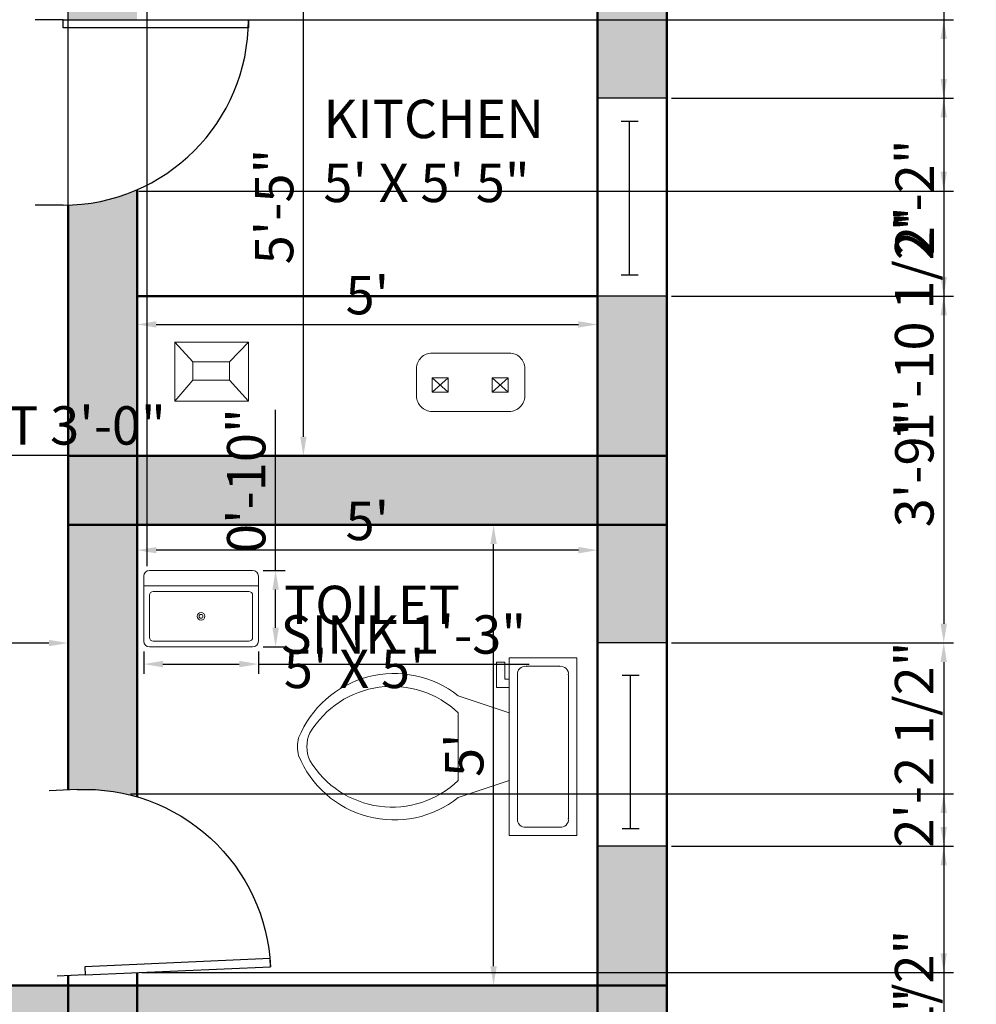
# Model space of a CAD drawing. Units: millimetres. Extents: x 2784 to 3697, y 603 to 1406.
# Tile 6 of 10: x 3091 to 3215, y 1077 to 1205. Entities that reach past the tile are written whole.
import ezdxf

# ---------------------------------------------------------------- set-up
doc = ezdxf.new("R2010")
doc.units = ezdxf.units.MM
for name, color, linetype, lineweight in [('A-ANNO-DIMS', 140, 'Continuous', 18), ('A-AREA-IDEN', 150, 'Continuous', 25), ('A-DOOR', 10, 'Continuous', 25), ('A-FLOR-FIXT', 8, 'Continuous', 18), ('A-FURN', 80, 'Continuous', 18), ('A-GLAZ', 30, 'Continuous', 25), ('A-WALL', 2, 'Continuous', 50), ('A-WALL-PATT', 8, 'Continuous', 13)]:
    doc.layers.add(name, color=color, linetype=linetype, lineweight=lineweight)
doc.styles.get("Standard").update_dxf_attribs({"font": 'arial.ttf'})
doc.dimstyles.new('ISO-25', dxfattribs={"dimtxt": 5, "dimasz": 2.5, "dimexe": 1.25, "dimexo": 0.625, "dimtad": 1, "dimdec": 0, "dimlunit": 3, "dimtxsty": 'Standard', "dimcen": 2.5, "dimadec": 0, "dimazin": 0, "dimtfac": 1, "dimtdec": 0, "dimtmove": 0, "dimatfit": 3, "dimfxl": 1, "dimarcsym": 0})

# ---------------------------------------------------------------- blocks, each defined once
blk = doc.blocks.new('*U2')
for p, q in [((0, 0), (0, -6)), ((40, 0), (40, -6))]:
    blk.add_line(p, q)
blk.add_lwpolyline([(0, 0), (0, 40), (1.75, 40), (1.75, 0)], close=True)
blk.add_arc((0, 0), 40, 0, 90)
blk = doc.blocks.new('*U5')
for p, q in [((0, 4), (0, 0)), ((36, 4), (36, 0)), ((0, 2), (36, 2))]:
    blk.add_line(p, q)
blk = doc.blocks.new('Toilet - top')
for p, q in [((9.5, -6), (9.5, -2)), ((-8, -8.5), (-8, -8)), ((-7, -8), (-7, -9.5)), ((-4, -8), (-6, -14)), ((4, -8), (6, -14)), ((-10, -8.5), (-8, -8.5)), ((-10, -9.5), (-10, -8.5)), ((-7, -9.5), (-10, -9.5)), ((4, -14), (-4, -14))]:
    blk.add_line(p, q)
blk.add_lwpolyline([(10.5, -8), (10.5, 0), (-10.5, 0), (-10.5, -8)], close=True)
for points in [[(8.5, -1), (-8.5, -1)], [(-9.5, -2), (-9.5, -6)], [(-8.5, -7), (8.5, -7)]]:
    blk.add_lwpolyline(points)
for centre, radius, start, end in [((-8.62, -1.88), 0.884, 81.8699, 188.1301), ((8.62, -1.88), 0.884, 351.8699, 98.1301), ((-8.62, -6.12), 0.884, 171.8699, 278.1301), ((8.62, -6.12), 0.884, 261.8699, 8.1301), ((3.52, -21.58), 12.17, 141.4691, 247.9714), ((4.2, -21.82), 11.33, 136.3677, 238.9468), ((-3.52, -21.58), 12.17, 292.0284, 38.5307), ((-4.2, -21.82), 11.33, 301.053, 43.6321), ((0, -27.88), 4, 245.7318, 294.2682), ((0, -29), 4, 254.8605, 285.1395)]:
    blk.add_arc(centre, radius, start, end)
blk = doc.blocks.new('Sink-single - 30 in top')
blk.add_line((-15, -3.999996), (15, -3.999996))
for points in [[(-13.5, 0), (13.5, 0)], [(-15, -18.499996), (-15, -1.5)], [(15, -1.5), (15, -18.499996)], [(-13.5, -17.499996), (-13.5, -6.499996)], [(-12.5, -5.499996), (12.5, -5.499996)], [(13.5, -6.499996), (13.5, -17.499996)], [(13.5, -19.999996), (-13.5, -19.999996)], [(12.5, -18.499996), (-12.5, -18.499996)]]:
    blk.add_lwpolyline(points)
for radius in [1, 0.5]:
    blk.add_circle((0, -11.999996), radius)
for centre, radius, start, end in [((-13.5, -1.5), 1.5, 90, 180), ((13.5, -1.5), 1.5, 0, 90), ((-12.5, -6.499996), 1, 90, 180), ((12.5, -6.499996), 1, 0, 90), ((-12.5, -17.499996), 1, 180, 270), ((12.5, -17.499996), 1, 270, 0), ((-13.5, -18.499996), 1.5, 180, 270), ((13.5, -18.499996), 1.5, 270, 0)]:
    blk.add_arc(centre, radius, start, end)
blk = doc.blocks.new('*D23')
at = {"layer": 'A-ANNO-DIMS', "color": 0, "lineweight": -2, "transparency": 16777216}
for p, q in [((3105.91, 1165.32), (3105.91, 1164.11)), ((3108.41, 1165.36), (3163.41, 1165.36)), ((3165.91, 1165.32), (3165.91, 1164.11))]:
    blk.add_line(p, q, dxfattribs=at)
at = {"layer": 'A-ANNO-DIMS', "color": 0, "transparency": 16777216}
for points in [[(3108.41, 1165.78), (3108.41, 1164.95), (3105.91, 1165.36)], [(3163.41, 1165.78), (3163.41, 1164.95), (3165.91, 1165.36)]]:
    blk.add_solid(points, dxfattribs=at)
at = {"layer": 'Defpoints', "color": 0, "transparency": 16777216}
for p in [(3105.91, 1165.95), (3165.91, 1165.95), (3165.91, 1165.36)]:
    blk.add_point(p, dxfattribs=at)
at = {"layer": 'A-ANNO-DIMS', "color": 0, "transparency": 16777216, "insert": (3135.91, 1168.53), "char_height": 5, "attachment_point": 5}
blk.add_mtext("5'", dxfattribs=at)
blk = doc.blocks.new('*D24')
at = {"layer": 'A-ANNO-DIMS', "color": 0, "lineweight": -2, "transparency": 16777216}
for p, q in [((3124.34, 1213.23), (3128.82, 1213.23)), ((3127.57, 1150.73), (3127.57, 1210.73)), ((3124.34, 1148.23), (3128.82, 1148.23))]:
    blk.add_line(p, q, dxfattribs=at)
at = {"layer": 'A-ANNO-DIMS', "color": 0, "transparency": 16777216}
for points in [[(3127.15, 1210.73), (3127.98, 1210.73), (3127.57, 1213.23)], [(3127.15, 1150.73), (3127.98, 1150.73), (3127.57, 1148.23)]]:
    blk.add_solid(points, dxfattribs=at)
at = {"layer": 'Defpoints', "color": 0, "transparency": 16777216}
for p in [(3123.72, 1213.23), (3127.57, 1213.23), (3123.72, 1148.23)]:
    blk.add_point(p, dxfattribs=at)
at = {"layer": 'A-ANNO-DIMS', "color": 0, "transparency": 16777216, "insert": (3124.4, 1180.73), "char_height": 5, "attachment_point": 5, "rotation": 90}
blk.add_mtext('5\'-5"', dxfattribs=at)
blk = doc.blocks.new('*D25')
at = {"layer": 'A-ANNO-DIMS', "color": 0, "lineweight": -2, "transparency": 16777216}
for p, q in [((3105.91, 1136.2), (3105.91, 1134.7)), ((3163.41, 1135.95), (3108.41, 1135.95)), ((3165.91, 1136.2), (3165.91, 1134.7))]:
    blk.add_line(p, q, dxfattribs=at)
at = {"layer": 'A-ANNO-DIMS', "color": 0, "transparency": 16777216}
for points in [[(3108.41, 1136.36), (3108.41, 1135.53), (3105.91, 1135.95)], [(3163.41, 1136.36), (3163.41, 1135.53), (3165.91, 1135.95)]]:
    blk.add_solid(points, dxfattribs=at)
at = {"layer": 'Defpoints', "color": 0, "transparency": 16777216}
for p in [(3105.91, 1136.83), (3165.91, 1136.83), (3105.91, 1135.95)]:
    blk.add_point(p, dxfattribs=at)
at = {"layer": 'A-ANNO-DIMS', "color": 0, "transparency": 16777216, "insert": (3135.91, 1139.11), "char_height": 5, "attachment_point": 5}
blk.add_mtext("5'", dxfattribs=at)
blk = doc.blocks.new('*D26')
at = {"layer": 'A-ANNO-DIMS', "color": 0, "lineweight": -2, "transparency": 16777216}
for p, q in [((3152.97, 1139.23), (3153.6, 1139.23)), ((3152.35, 1081.73), (3152.35, 1136.73)), ((3152.97, 1079.23), (3153.6, 1079.23))]:
    blk.add_line(p, q, dxfattribs=at)
at = {"layer": 'A-ANNO-DIMS', "color": 0, "transparency": 16777216}
for points in [[(3151.93, 1136.73), (3152.77, 1136.73), (3152.35, 1139.23)], [(3151.93, 1081.73), (3152.77, 1081.73), (3152.35, 1079.23)]]:
    blk.add_solid(points, dxfattribs=at)
at = {"layer": 'Defpoints', "color": 0, "transparency": 16777216}
for p in [(3152.35, 1139.23), (3152.35, 1139.23), (3152.35, 1079.23)]:
    blk.add_point(p, dxfattribs=at)
at = {"layer": 'A-ANNO-DIMS', "color": 0, "transparency": 16777216, "insert": (3149.18, 1109.23), "char_height": 5, "attachment_point": 5, "rotation": 90}
blk.add_mtext("5'", dxfattribs=at)
blk = doc.blocks.new('*D36')
at = {"layer": 'A-ANNO-DIMS', "color": 0, "lineweight": -2, "transparency": 16777216}
for p, q in [((2971.91, 1166.33), (2971.91, 1122.59)), ((3096.91, 1166.33), (3096.91, 1122.59)), ((3094.41, 1123.84), (2974.41, 1123.84))]:
    blk.add_line(p, q, dxfattribs=at)
at = {"layer": 'A-ANNO-DIMS', "color": 0, "transparency": 16777216}
for points in [[(2974.41, 1124.26), (2974.41, 1123.43), (2971.91, 1123.84)], [(3094.41, 1124.26), (3094.41, 1123.43), (3096.91, 1123.84)]]:
    blk.add_solid(points, dxfattribs=at)
at = {"layer": 'Defpoints', "color": 0, "transparency": 16777216}
for p in [(2971.91, 1166.96), (3096.91, 1166.96), (2971.91, 1123.84)]:
    blk.add_point(p, dxfattribs=at)
at = {"layer": 'A-ANNO-DIMS', "color": 0, "transparency": 16777216, "insert": (3034.41, 1127.02), "char_height": 5, "attachment_point": 5}
blk.add_mtext('10\'-5"', dxfattribs=at)
blk = doc.blocks.new('*D66')
at = {"layer": 'A-ANNO-DIMS', "color": 0, "lineweight": -2, "transparency": 16777216}
for p, q in [((3106.77, 1122.72), (3106.77, 1119.85)), ((3121.71, 1122.72), (3121.71, 1119.85)), ((3109.27, 1121.1), (3119.21, 1121.1)), ((3121.71, 1121.1), (3156.97, 1121.1))]:
    blk.add_line(p, q, dxfattribs=at)
at = {"layer": 'A-ANNO-DIMS', "color": 0, "transparency": 16777216}
for points in [[(3109.27, 1121.52), (3109.27, 1120.68), (3106.77, 1121.1)], [(3119.21, 1121.52), (3119.21, 1120.68), (3121.71, 1121.1)]]:
    blk.add_solid(points, dxfattribs=at)
at = {"layer": 'Defpoints', "color": 0, "transparency": 16777216}
for p in [(3106.77, 1123.34), (3121.71, 1123.34), (3121.71, 1121.1)]:
    blk.add_point(p, dxfattribs=at)
at = {"layer": 'A-ANNO-DIMS', "color": 0, "transparency": 16777216, "insert": (3140.59, 1124.31), "char_height": 5, "attachment_point": 5}
blk.add_mtext('SINK 1\'-3"', dxfattribs=at)
blk = doc.blocks.new('*D67')
at = {"layer": 'A-ANNO-DIMS', "color": 0, "lineweight": -2, "transparency": 16777216}
for p, q in [((3123.95, 1133.3), (3123.95, 1154.22)), ((3122.33, 1133.3), (3125.2, 1133.3)), ((3123.95, 1125.84), (3123.95, 1130.8)), ((3122.33, 1123.34), (3125.2, 1123.34))]:
    blk.add_line(p, q, dxfattribs=at)
at = {"layer": 'A-ANNO-DIMS', "color": 0, "transparency": 16777216}
for points in [[(3123.53, 1130.8), (3124.37, 1130.8), (3123.95, 1133.3)], [(3123.53, 1125.84), (3124.37, 1125.84), (3123.95, 1123.34)]]:
    blk.add_solid(points, dxfattribs=at)
at = {"layer": 'Defpoints', "color": 0, "transparency": 16777216}
for p in [(3121.71, 1133.3), (3123.95, 1133.3), (3121.71, 1123.34)]:
    blk.add_point(p, dxfattribs=at)
at = {"layer": 'A-ANNO-DIMS', "color": 0, "transparency": 16777216, "insert": (3120.77, 1145.01), "char_height": 5, "attachment_point": 5, "rotation": 90}
blk.add_mtext('0\'-10"', dxfattribs=at)
blk = doc.blocks.new('*D74')
at = {"layer": 'A-ANNO-DIMS', "color": 0, "lineweight": -2, "transparency": 16777216}
for p, q in [((3016.17, 1153.13), (3016.17, 1147.09)), ((3052.27, 1153.13), (3052.27, 1147.09)), ((3018.67, 1148.34), (3049.77, 1148.34)), ((3052.27, 1148.34), (3110.98, 1148.34))]:
    blk.add_line(p, q, dxfattribs=at)
at = {"layer": 'A-ANNO-DIMS', "color": 0, "transparency": 16777216}
for points in [[(3018.67, 1148.76), (3018.67, 1147.92), (3016.17, 1148.34)], [(3049.77, 1148.76), (3049.77, 1147.92), (3052.27, 1148.34)]]:
    blk.add_solid(points, dxfattribs=at)
at = {"layer": 'Defpoints', "color": 0, "transparency": 16777216}
for p in [(3016.17, 1153.76), (3052.27, 1153.76), (3052.27, 1148.34)]:
    blk.add_point(p, dxfattribs=at)
at = {"layer": 'A-ANNO-DIMS', "color": 0, "transparency": 16777216, "insert": (3082.87, 1151.55), "char_height": 5, "attachment_point": 5}
blk.add_mtext('DINING SET 3\'-0"', dxfattribs=at)
blk = doc.blocks.new('*D93')
at = {"layer": 'A-ANNO-DIMS', "color": 0, "lineweight": -2, "transparency": 16777216}
for p, q in [((3175.53, 1266.65), (3212.26, 1266.65)), ((3211.01, 1264.15), (3211.01, 1197.33)), ((3175.53, 1194.83), (3212.26, 1194.83))]:
    blk.add_line(p, q, dxfattribs=at)
at = {"layer": 'A-ANNO-DIMS', "color": 0, "transparency": 16777216}
for points in [[(3210.59, 1264.15), (3211.42, 1264.15), (3211.01, 1266.65)], [(3210.59, 1197.33), (3211.42, 1197.33), (3211.01, 1194.83)]]:
    blk.add_solid(points, dxfattribs=at)
at = {"layer": 'Defpoints', "color": 0, "transparency": 16777216}
for p in [(3174.91, 1266.65), (3174.91, 1194.83), (3211.01, 1194.83)]:
    blk.add_point(p, dxfattribs=at)
at = {"layer": 'A-ANNO-DIMS', "color": 0, "transparency": 16777216, "insert": (3207.83, 1230.74), "char_height": 5, "attachment_point": 5, "rotation": 90}
blk.add_mtext('6\'-0"', dxfattribs=at)
blk = doc.blocks.new('*D94')
at = {"layer": 'A-ANNO-DIMS', "color": 0, "lineweight": -2, "transparency": 16777216}
for p, q in [((3175.53, 1194.83), (3212.26, 1194.83)), ((3211.01, 1192.33), (3211.01, 1171.56)), ((3175.53, 1169.06), (3212.26, 1169.06))]:
    blk.add_line(p, q, dxfattribs=at)
at = {"layer": 'A-ANNO-DIMS', "color": 0, "transparency": 16777216}
for points in [[(3210.59, 1192.33), (3211.42, 1192.33), (3211.01, 1194.83)], [(3210.59, 1171.56), (3211.42, 1171.56), (3211.01, 1169.06)]]:
    blk.add_solid(points, dxfattribs=at)
at = {"layer": 'Defpoints', "color": 0, "transparency": 16777216}
for p in [(3174.91, 1194.83), (3174.91, 1169.06), (3211.01, 1169.06)]:
    blk.add_point(p, dxfattribs=at)
at = {"layer": 'A-ANNO-DIMS', "color": 0, "transparency": 16777216, "insert": (3207.87, 1181.94), "char_height": 5, "attachment_point": 5, "rotation": 90}
blk.add_mtext('2\'-2"', dxfattribs=at)
blk = doc.blocks.new('*D95')
at = {"layer": 'A-ANNO-DIMS', "color": 0, "lineweight": -2, "transparency": 16777216}
for p, q in [((3175.53, 1169.06), (3212.26, 1169.06)), ((3211.01, 1166.56), (3211.01, 1126.36)), ((3175.53, 1123.86), (3212.26, 1123.86))]:
    blk.add_line(p, q, dxfattribs=at)
at = {"layer": 'A-ANNO-DIMS', "color": 0, "transparency": 16777216}
for points in [[(3210.59, 1166.56), (3211.42, 1166.56), (3211.01, 1169.06)], [(3210.59, 1126.36), (3211.42, 1126.36), (3211.01, 1123.86)]]:
    blk.add_solid(points, dxfattribs=at)
at = {"layer": 'Defpoints', "color": 0, "transparency": 16777216}
for p in [(3174.91, 1169.06), (3174.91, 1123.86), (3211.01, 1123.86)]:
    blk.add_point(p, dxfattribs=at)
at = {"layer": 'A-ANNO-DIMS', "color": 0, "transparency": 16777216, "insert": (3207.83, 1146.46), "char_height": 5, "attachment_point": 5, "rotation": 90}
blk.add_mtext('3\'-9"', dxfattribs=at)
blk = doc.blocks.new('*D96')
at = {"layer": 'A-ANNO-DIMS', "color": 0, "lineweight": -2, "transparency": 16777216}
for p, q in [((3175.53, 1123.86), (3212.26, 1123.86)), ((3211.01, 1121.36), (3211.01, 1099.87)), ((3175.53, 1097.37), (3212.26, 1097.37))]:
    blk.add_line(p, q, dxfattribs=at)
at = {"layer": 'A-ANNO-DIMS', "color": 0, "transparency": 16777216}
for points in [[(3210.59, 1121.36), (3211.42, 1121.36), (3211.01, 1123.86)], [(3210.59, 1099.87), (3211.42, 1099.87), (3211.01, 1097.37)]]:
    blk.add_solid(points, dxfattribs=at)
at = {"layer": 'Defpoints', "color": 0, "transparency": 16777216}
for p in [(3174.91, 1123.86), (3174.91, 1097.37), (3211.01, 1097.37)]:
    blk.add_point(p, dxfattribs=at)
at = {"layer": 'A-ANNO-DIMS', "color": 0, "transparency": 16777216, "insert": (3207.8, 1110.61), "char_height": 5, "attachment_point": 5, "rotation": 90}
blk.add_mtext('2\'-2 1/2"', dxfattribs=at)
blk = doc.blocks.new('*D97')
at = {"layer": 'A-ANNO-DIMS', "color": 0, "lineweight": -2, "transparency": 16777216}
for p, q in [((3175.53, 1097.37), (3212.26, 1097.37)), ((3211.01, 1094.87), (3211.01, 1051.27)), ((3175.53, 1048.77), (3212.26, 1048.77))]:
    blk.add_line(p, q, dxfattribs=at)
at = {"layer": 'A-ANNO-DIMS', "color": 0, "transparency": 16777216}
for points in [[(3210.59, 1094.87), (3211.42, 1094.87), (3211.01, 1097.37)], [(3210.59, 1051.27), (3211.42, 1051.27), (3211.01, 1048.77)]]:
    blk.add_solid(points, dxfattribs=at)
at = {"layer": 'Defpoints', "color": 0, "transparency": 16777216}
for p in [(3174.91, 1097.37), (3174.91, 1048.77), (3211.01, 1048.77)]:
    blk.add_point(p, dxfattribs=at)
at = {"layer": 'A-ANNO-DIMS', "color": 0, "transparency": 16777216, "insert": (3207.8, 1073.07), "char_height": 5, "attachment_point": 5, "rotation": 90}
blk.add_mtext('4\'-0 1/2"', dxfattribs=at)
blk = doc.blocks.new('*D106')
at = {"layer": 'A-ANNO-DIMS', "color": 0, "lineweight": -2, "transparency": 16777216}
for p, q in [((3106.53, 1205.07), (3212.26, 1205.07)), ((3211.01, 1202.57), (3211.01, 1185.25)), ((3106.12, 1182.75), (3212.26, 1182.75)), ((3211.01, 1182.75), (3211.01, 1150.64))]:
    blk.add_line(p, q, dxfattribs=at)
at = {"layer": 'A-ANNO-DIMS', "color": 0, "transparency": 16777216}
for points in [[(3210.59, 1202.57), (3211.42, 1202.57), (3211.01, 1205.07)], [(3210.59, 1185.25), (3211.42, 1185.25), (3211.01, 1182.75)]]:
    blk.add_solid(points, dxfattribs=at)
at = {"layer": 'Defpoints', "color": 0, "transparency": 16777216}
for p in [(3105.91, 1205.07), (3105.49, 1182.75), (3211.01, 1182.75)]:
    blk.add_point(p, dxfattribs=at)
at = {"layer": 'A-ANNO-DIMS', "color": 0, "transparency": 16777216, "insert": (3207.8, 1165.44), "char_height": 5, "attachment_point": 5, "rotation": 90}
blk.add_mtext('1\'-10 1/2"', dxfattribs=at)
blk = doc.blocks.new('*D107')
at = {"layer": 'A-ANNO-DIMS', "color": 0, "lineweight": -2, "transparency": 16777216}
for p, q in [((3105.04, 1104.19), (3212.26, 1104.19)), ((3211.01, 1101.69), (3211.01, 1083.41)), ((3106.53, 1080.91), (3212.26, 1080.91)), ((3211.01, 1080.91), (3211.01, 1048.8))]:
    blk.add_line(p, q, dxfattribs=at)
at = {"layer": 'A-ANNO-DIMS', "color": 0, "transparency": 16777216}
for points in [[(3210.59, 1101.69), (3211.42, 1101.69), (3211.01, 1104.19)], [(3210.59, 1083.41), (3211.42, 1083.41), (3211.01, 1080.91)]]:
    blk.add_solid(points, dxfattribs=at)
at = {"layer": 'Defpoints', "color": 0, "transparency": 16777216}
for p in [(3104.41, 1104.19), (3105.91, 1080.91), (3211.01, 1080.91)]:
    blk.add_point(p, dxfattribs=at)
at = {"layer": 'A-ANNO-DIMS', "color": 0, "transparency": 16777216, "insert": (3207.8, 1063.61), "char_height": 5, "attachment_point": 5, "rotation": 90}
blk.add_mtext('1\'-11 1/2"', dxfattribs=at)
blk = doc.blocks.new('*D108')
at = {"layer": 'A-ANNO-DIMS', "color": 0, "lineweight": -2, "transparency": 16777216}
for p, q in [((3165.91, 1169.69), (3165.91, 1393.58)), ((3174.91, 1169.69), (3174.91, 1393.58)), ((3168.41, 1392.33), (3172.41, 1392.33)), ((3174.91, 1392.33), (3191.95, 1392.33))]:
    blk.add_line(p, q, dxfattribs=at)
at = {"layer": 'A-ANNO-DIMS', "color": 0, "transparency": 16777216}
for points in [[(3168.41, 1392.75), (3168.41, 1391.91), (3165.91, 1392.33)], [(3172.41, 1392.75), (3172.41, 1391.91), (3174.91, 1392.33)]]:
    blk.add_solid(points, dxfattribs=at)
at = {"layer": 'Defpoints', "color": 0, "transparency": 16777216}
for p in [(3174.91, 1392.33), (3165.91, 1169.06), (3174.91, 1169.06)]:
    blk.add_point(p, dxfattribs=at)
at = {"layer": 'A-ANNO-DIMS', "color": 0, "transparency": 16777216, "insert": (3184.68, 1395.51), "char_height": 5, "attachment_point": 5}
blk.add_mtext('0\'-9"', dxfattribs=at)
blk = doc.blocks.new('*D109')
at = {"layer": 'A-ANNO-DIMS', "color": 0, "lineweight": -2, "transparency": 16777216}
for p, q in [((3096.91, 1139.86), (3096.91, 1393.58)), ((3107.23, 1133.86), (3107.23, 1393.58)), ((3099.41, 1392.33), (3104.73, 1392.33)), ((3107.23, 1392.33), (3139.81, 1392.33))]:
    blk.add_line(p, q, dxfattribs=at)
at = {"layer": 'A-ANNO-DIMS', "color": 0, "transparency": 16777216}
for points in [[(3099.41, 1392.75), (3099.41, 1391.91), (3096.91, 1392.33)], [(3104.73, 1392.75), (3104.73, 1391.91), (3107.23, 1392.33)]]:
    blk.add_solid(points, dxfattribs=at)
at = {"layer": 'Defpoints', "color": 0, "transparency": 16777216}
for p in [(3107.23, 1392.33), (3096.91, 1139.23), (3107.23, 1133.24)]:
    blk.add_point(p, dxfattribs=at)
at = {"layer": 'A-ANNO-DIMS', "color": 0, "transparency": 16777216, "insert": (3124.77, 1395.54), "char_height": 5, "attachment_point": 5}
blk.add_mtext('0\'-10 1/2"', dxfattribs=at)

msp = doc.modelspace()

# ---------------------------------------------------------------- hatches: boundary and pattern name
at = {"layer": 'A-FLOR-FIXT'}
h = msp.add_hatch(color=256, dxfattribs=at)
h.dxf.hatch_style = 1
h.paths.add_polyline_path([(3174.91, 1169.06), (3165.91, 1169.06), (3165.91, 1148.23), (3174.91, 1148.23)])
at = {"layer": 'A-WALL-PATT'}
h = msp.add_hatch(color=256, dxfattribs=at)
h.dxf.hatch_style = 1
h.paths.add_polyline_path([(2869.53, 1356.23), (2839.91, 1356.23), (2839.91, 1347.23), (2869.53, 1347.23)])
h.paths.add_polyline_path([(2839.91, 1356.23), (2830.91, 1356.23), (2830.91, 1347.23), (2839.91, 1347.23)])
h.paths.add_polyline_path([(2839.91, 1347.23), (2830.91, 1347.23), (2830.91, 1314.23), (2839.91, 1314.23)])
h.paths.add_polyline_path([(2839.91, 1268.19), (2830.91, 1268.19), (2830.91, 1222.23), (2839.91, 1222.23)])
h.paths.add_polyline_path([(2839.91, 1222.23), (2830.91, 1222.23), (2830.91, 1213.23), (2839.91, 1213.23)])
h.paths.add_polyline_path([(2962.91, 1222.23), (2839.91, 1222.23), (2839.91, 1213.23), (2962.91, 1213.23)])
h.paths.add_polyline_path([(2971.91, 1222.23), (2962.91, 1222.23), (2962.91, 1213.23), (2971.91, 1213.23)])
h.paths.add_polyline_path([(2971.91, 1263.23), (2962.91, 1263.23), (2962.91, 1254.23), (2971.91, 1254.23)])
h.paths.add_polyline_path([(2971.91, 1347.23), (2962.91, 1347.23), (2962.91, 1263.23), (2971.91, 1263.23)])
h.paths.add_polyline_path([(2971.91, 1356.23), (2962.91, 1356.23), (2962.91, 1347.23), (2971.91, 1347.23)])
h.paths.add_polyline_path([(2962.91, 1356.23), (2913.7, 1356.23), (2913.7, 1347.23), (2962.91, 1347.23)])
h.paths.add_polyline_path([(2982.62, 1356.23), (2971.91, 1356.23), (2971.91, 1347.23), (2982.62, 1347.23)])
h.paths.add_polyline_path([(3019.91, 1356.23), (3004.44, 1356.23), (3004.44, 1347.23), (3019.91, 1347.23)])
h.paths.add_polyline_path([(3028.91, 1356.23), (3019.91, 1356.23), (3019.91, 1347.23), (3028.91, 1347.23)])
h.paths.add_polyline_path([(3028.91, 1347.23), (3019.91, 1347.23), (3019.91, 1287.35, -0.06506), (3026.12, 1288.16), (3028.91, 1288.16)])
h.paths.add_polyline_path([(3019.91, 1263.23), (2971.91, 1263.23), (2971.91, 1254.23), (3019.91, 1254.23)])
h.paths.add_polyline_path([(3028.91, 1263.23), (3019.91, 1263.23), (3019.91, 1254.23), (3028.91, 1254.23)])
h.paths.add_polyline_path([(3028.91, 1254.23), (3019.91, 1254.23), (3019.91, 1222.23), (3028.91, 1222.23)])
h.paths.add_polyline_path([(3028.91, 1222.23), (3019.91, 1222.23), (3019.91, 1213.23), (3028.91, 1213.23)])
h.paths.add_polyline_path([(3165.91, 1222.23), (3060.65, 1222.23, -0.056956), (3061.45, 1215.23), (3061.45, 1213.23), (3165.91, 1213.23)])
h.paths.add_polyline_path([(3080.34, 1356.23), (3028.91, 1356.23), (3028.91, 1347.23), (3080.34, 1347.23)])
h.paths.add_polyline_path([(3174.91, 1347.23), (3165.91, 1347.23), (3165.91, 1311.28), (3174.91, 1311.28)])
h.paths.add_polyline_path([(3174.91, 1356.23), (3165.91, 1356.23), (3165.91, 1347.23), (3174.91, 1347.23)])
h.paths.add_polyline_path([(3165.91, 1356.23), (3123.1, 1356.23), (3123.1, 1347.23), (3165.91, 1347.23)])
h.paths.add_polyline_path([(3174.91, 1266.65), (3165.91, 1266.65), (3165.91, 1222.23), (3174.91, 1222.23)])
h.paths.add_polyline_path([(3174.91, 1222.23), (3165.91, 1222.23), (3165.91, 1213.23), (3174.91, 1213.23)])
h.paths.add_polyline_path([(3174.91, 1213.23), (3165.91, 1213.23), (3165.91, 1194.83), (3174.91, 1194.83)])
h.paths.add_polyline_path([(3105.91, 1182.92, -0.096276), (3096.91, 1180.92), (3096.91, 1148.23), (3105.91, 1148.23)])
h.paths.add_polyline_path([(3105.91, 1213.23), (3096.91, 1213.23), (3096.91, 1205.07), (3105.91, 1205.07)])
h.paths.add_polyline_path([(2971.91, 1213.23), (2962.91, 1213.23), (2962.91, 1161.09), (2971.91, 1161.09)])
h.paths.add_polyline_path([(2839.91, 1213.23), (2830.91, 1213.23), (2830.91, 1157.46), (2839.91, 1157.46)])
h.paths.add_polyline_path([(2839.91, 1108.88), (2830.91, 1108.88), (2830.91, 1042.23), (2839.91, 1042.23)])
h.paths.add_polyline_path([(2839.91, 1042.23), (2830.91, 1042.23), (2830.91, 1033.23), (2839.91, 1033.23)])
h.paths.add_polyline_path([(2881.91, 1042.23), (2839.91, 1042.23), (2839.91, 1033.23), (2881.91, 1033.23)])
h.paths.add_polyline_path([(2996.91, 1042.23), (2890.91, 1042.23), (2890.91, 1033.23), (2996.91, 1033.23)])
h.paths.add_polyline_path([(2890.91, 1042.23), (2881.91, 1042.23), (2881.91, 1033.23), (2890.91, 1033.23)])
h.paths.add_polyline_path([(2890.91, 1033.23), (2881.91, 1033.23), (2881.91, 984.23), (2890.91, 984.23)])
h.paths.add_polyline_path([(2839.91, 1033.23), (2830.91, 1033.23), (2830.91, 984.23), (2839.91, 984.23)])
h.paths.add_polyline_path([(2839.91, 984.23), (2830.91, 984.23), (2830.91, 975.23), (2839.91, 975.23)])
h.paths.add_polyline_path([(2881.91, 984.23), (2854.14, 984.23, -0.154991), (2857.05, 975.23), (2881.91, 975.23)])
h.paths.add_polyline_path([(2890.91, 984.23), (2881.91, 984.23), (2881.91, 975.23), (2890.91, 975.23)])
h.paths.add_polyline_path([(2900.85, 984.23), (2890.91, 984.23), (2890.91, 975.23), (2900.85, 975.23), (2900.85, 975.78)])
h.paths.add_polyline_path([(2996.91, 984.23), (2923.49, 984.23, -0.089525), (2925.01, 975.78), (2925.01, 975.23), (2996.91, 975.23)])
h.paths.add_polyline_path([(3165.91, 984.23), (3005.91, 984.23), (3005.91, 975.23), (3165.91, 975.23)])
h.paths.add_polyline_path([(3005.91, 1033.23), (2996.91, 1033.23), (2996.91, 984.23), (3005.91, 984.23)])
h.paths.add_polyline_path([(3005.91, 984.23), (2996.91, 984.23), (2996.91, 975.23), (3005.91, 975.23)])
h.paths.add_polyline_path([(3005.91, 1042.23), (2996.91, 1042.23), (2996.91, 1033.23), (3005.91, 1033.23)])
h.paths.add_polyline_path([(3096.91, 1079.23), (2971.91, 1079.23), (2971.91, 1070.23), (3096.91, 1070.23)])
h.paths.add_polyline_path([(2971.91, 1079.23), (2962.91, 1079.23), (2962.91, 1070.23), (2971.91, 1070.23)])
h.paths.add_polyline_path([(2971.91, 1070.23), (2962.91, 1070.23), (2962.91, 1060.28, -0.115005), (2971.91, 1066.55)])
h.paths.add_polyline_path([(2971.91, 1105.54), (2962.91, 1105.54), (2962.91, 1079.23), (2971.91, 1079.23)])
h.paths.add_polyline_path([(3165.91, 1079.23), (3105.91, 1079.23), (3105.91, 1070.23), (3165.91, 1070.23)])
h.paths.add_polyline_path([(3105.91, 1079.23), (3096.91, 1079.23), (3096.91, 1070.23), (3105.91, 1070.23)])
h.paths.add_polyline_path([(3105.91, 1148.23), (3096.91, 1148.23), (3096.91, 1139.23), (3105.91, 1139.23)])
h.paths.add_polyline_path([(3105.91, 1139.23), (3096.91, 1139.23), (3096.91, 1104.7), (3098.08, 1104.75, -0.08216), (3105.91, 1103.81)])
h.paths.add_polyline_path([(3165.91, 1148.23), (3105.91, 1148.23), (3105.91, 1139.23), (3165.91, 1139.23)])
h.paths.add_polyline_path([(3174.91, 1148.23), (3165.91, 1148.23), (3165.91, 1139.23), (3174.91, 1139.23)])
h.paths.add_polyline_path([(3174.91, 1139.23), (3165.91, 1139.23), (3165.91, 1123.86), (3174.91, 1123.86)])
h.paths.add_polyline_path([(3174.91, 1097.37), (3165.91, 1097.37), (3165.91, 1079.23), (3174.91, 1079.23)])
h.paths.add_polyline_path([(3174.91, 1079.23), (3165.91, 1079.23), (3165.91, 1070.23), (3174.91, 1070.23)])
h.paths.add_polyline_path([(3174.91, 1070.23), (3165.91, 1070.23), (3165.91, 1048.77), (3174.91, 1048.77)])
h.paths.add_polyline_path([(3174.91, 1002.74), (3165.91, 1002.74), (3165.91, 984.23), (3174.91, 984.23)])
h.paths.add_polyline_path([(3174.91, 984.23), (3165.91, 984.23), (3165.91, 975.23), (3174.91, 975.23)])
h.paths.add_polyline_path([(3174.91, 975.23), (3165.91, 975.23), (3165.91, 725.23), (3174.91, 725.23)])
h.paths.add_polyline_path([(2839.91, 975.23), (2830.91, 975.23), (2830.91, 725.23), (2839.91, 725.23)])
h.paths.add_polyline_path([(3165.91, 725.23), (2839.91, 725.23), (2839.91, 716.23), (3165.91, 716.23)])
h.paths.add_polyline_path([(3174.91, 725.23), (3165.91, 725.23), (3165.91, 716.23), (3174.91, 716.23)])
h.paths.add_polyline_path([(2839.91, 725.23), (2830.91, 725.23), (2830.91, 716.23), (2839.91, 716.23)])

# ---------------------------------------------------------------- linework, layer by layer
at = {"layer": 'A-FURN'}
for p, q in [((3113.17, 1160.47), (3110.8, 1163.06)), ((3117.96, 1160.47), (3120.42, 1163.06)), ((3113.17, 1158.11), (3110.8, 1155.35)), ((3117.96, 1158.11), (3120.42, 1155.35)), ((3146.45, 1156.55), (3144.36, 1158.41)), ((3144.36, 1156.55), (3146.45, 1158.41)), ((3152.18, 1158.41), (3154.26, 1156.55)), ((3152.18, 1156.55), (3154.26, 1158.41))]:
    msp.add_line(p, q, dxfattribs=at)
for points in [[(3110.8, 1163.06), (3120.42, 1163.06), (3120.42, 1155.35), (3110.8, 1155.35)], [(3113.17, 1160.47), (3117.96, 1160.47), (3117.96, 1158.11), (3113.17, 1158.11)], [(3144.36, 1158.41), (3146.45, 1158.41), (3146.45, 1156.55), (3144.36, 1156.55)], [(3152.18, 1158.41), (3154.26, 1158.41), (3154.26, 1156.55), (3152.18, 1156.55)]]:
    msp.add_lwpolyline(points, close=True, dxfattribs=at)
msp.add_lwpolyline([(3144.32, 1161.63), (3154.42, 1161.63, -0.414214), (3156.42, 1159.63), (3156.42, 1156.02, -0.414214), (3154.42, 1154.02), (3144.32, 1154.02, -0.414214), (3142.32, 1156.02), (3142.32, 1159.63, -0.414214)], format="xyb", close=True, dxfattribs=at)
at = {"layer": 'A-GLAZ'}
for p, q in [((3174.91, 1194.83), (3165.91, 1194.83)), ((3174.91, 1169.06), (3165.91, 1169.06)), ((3174.91, 1123.86), (3165.91, 1123.86)), ((3174.91, 1097.37), (3165.91, 1097.37))]:
    msp.add_line(p, q, dxfattribs=at)
at = {"layer": 'A-WALL'}
for p, q in [((3165.91, 1213.23), (3165.91, 643.6)), ((3174.91, 1213.23), (3174.91, 643.6)), ((3105.91, 1182.92), (3105.91, 1103.81)), ((3096.91, 1180.92), (3096.91, 1104.7)), ((3165.91, 1169.06), (3105.91, 1169.06)), ((3096.91, 1148.23), (3174.91, 1148.23)), ((3096.91, 1139.23), (3174.91, 1139.23)), ((3096.91, 1080.52), (3096.91, 1070.23)), ((3105.91, 1080.91), (3105.91, 1070.23)), ((2962.91, 1079.23), (3174.91, 1079.23))]:
    msp.add_line(p, q, dxfattribs=at)

# ---------------------------------------------------------------- block references
at = {"layer": 'A-DOOR', "yscale": 0.6041131756153701, "zscale": 0.6041131756153701}
for p, xscale, rotation in [((3096.25, 1205.07), 0.6041131756153701, 270), ((3099.13, 1080.61), -0.6041131756153701, 272.5062906382857)]:
    msp.add_blockref('*U2', p, dxfattribs=dict(at, xscale=xscale, rotation=rotation))
at = {"layer": 'A-FLOR-FIXT', "xscale": 0.4978519308129675, "yscale": 0.4978519308129675, "zscale": 0.4978519308129675}
msp.add_blockref('Sink-single - 30 in top', (3114.24, 1133.3), dxfattribs=at)
at = {"layer": 'A-FLOR-FIXT', "xscale": 1.103188224763309, "yscale": 1.103188224763309, "zscale": 1.103188224763309, "rotation": 270}
msp.add_blockref('Toilet - top', (3163.2, 1110.33), dxfattribs=at)
at = {"layer": 'A-GLAZ', "xscale": 0.5552882983770857, "yscale": 0.5552882983770857, "zscale": 0.5552882983770857, "rotation": 90}
for p in [(3171.18, 1171.84), (3171.32, 1099.66)]:
    msp.add_blockref('*U5', p, dxfattribs=at)

# ---------------------------------------------------------------- texts
at = {"layer": 'A-AREA-IDEN', "char_height": 5, "attachment_point": 1}
for s, width, insert in [('KITCHEN \\P5\' X 5\' 5"', 28.5828, (3130.18, 1194.64)), ("TOILET \\P5' X 5'", 22.2139, (3125.03, 1131.31))]:
    msp.add_mtext_dynamic_manual_height_columns(s, width=width, gutter_width=12.5, heights=[0], dxfattribs=dict(at, insert=insert))

# ---------------------------------------------------------------- dimensions: what is measured, and where the dimension line sits
at = {"layer": 'A-ANNO-DIMS'}
for base, p1, p2, override, picture, middle in [((3107.23, 1392.33), (3096.91, 1139.23), (3107.23, 1133.24), {"dimdec": 1, "dimlfac": 1, "dimrnd": 0, "dimzin": 1, "dimdsep": 46, "dimlunit": 4, "dimfrac": 2}, '*D109', (3124.77, 1395.54)), ((3174.91, 1392.33), (3165.91, 1169.06), (3174.91, 1169.06), {"dimdec": 1, "dimlfac": 1, "dimrnd": 0, "dimzin": 1, "dimdsep": 46, "dimlunit": 4, "dimfrac": 2}, '*D108', (3184.68, 1395.51)), ((3165.91, 1165.36), (3105.91, 1165.95), (3165.91, 1165.95), {"dimclrd": 0, "dimclre": 0, "dimclrt": 0}, '*D23', (3135.91, 1168.53)), ((2971.91, 1123.84), (3096.91, 1166.96), (2971.91, 1166.96), {"dimclrd": 0, "dimclre": 0, "dimclrt": 0}, '*D36', (3034.41, 1127.02)), ((3105.91, 1135.95), (3165.91, 1136.83), (3105.91, 1136.83), {"dimclrd": 0, "dimclre": 0, "dimclrt": 0}, '*D25', (3135.91, 1139.11))]:
    dim = msp.add_linear_dim(base=base, p1=p1, p2=p2, dimstyle='ISO-25', override=override, dxfattribs=at)
    dim.commit()
    dim.dimension.update_dxf_attribs({"geometry": picture, "text_midpoint": middle})
for base, p1, p2, override, picture, middle in [((3211.01, 1194.83), (3174.91, 1266.65), (3174.91, 1194.83), {"dimdec": 1, "dimlfac": 1, "dimrnd": 0, "dimzin": 1, "dimdsep": 46, "dimlunit": 4, "dimfrac": 2}, '*D93', (3207.83, 1230.74)), ((3127.57, 1213.23), (3123.72, 1148.23), (3123.72, 1213.23), {"dimclrd": 0, "dimclre": 0, "dimclrt": 0}, '*D24', (3124.4, 1180.73)), ((3211.01, 1182.75), (3105.91, 1205.07), (3105.49, 1182.75), {"dimdec": 1, "dimlfac": 1, "dimrnd": 0, "dimzin": 1, "dimdsep": 46, "dimlunit": 4, "dimfrac": 2}, '*D106', (3207.8, 1165.44)), ((3211.01, 1169.06), (3174.91, 1194.83), (3174.91, 1169.06), {"dimdec": 1, "dimlfac": 1, "dimrnd": 0, "dimzin": 1, "dimdsep": 46, "dimlunit": 4, "dimfrac": 2}, '*D94', (3207.87, 1181.94)), ((3211.01, 1123.86), (3174.91, 1169.06), (3174.91, 1123.86), {"dimdec": 1, "dimlfac": 1, "dimrnd": 0, "dimzin": 1, "dimdsep": 46, "dimlunit": 4, "dimfrac": 2}, '*D95', (3207.83, 1146.46)), ((3123.95, 1133.3), (3121.71, 1123.34), (3121.71, 1133.3), {"dimdec": 1, "dimrnd": 0, "dimzin": 1, "dimlunit": 4, "dimfrac": 2}, '*D67', (3120.77, 1145.01)), ((3152.35, 1139.23), (3152.35, 1079.23), (3152.35, 1139.23), {"dimclrd": 0, "dimclre": 0, "dimclrt": 0}, '*D26', (3149.18, 1109.23)), ((3211.01, 1097.37), (3174.91, 1123.86), (3174.91, 1097.37), {"dimdec": 1, "dimlfac": 1, "dimrnd": 0, "dimzin": 1, "dimdsep": 46, "dimlunit": 4, "dimfrac": 2}, '*D96', (3207.8, 1110.61)), ((3211.01, 1080.91), (3104.41, 1104.19), (3105.91, 1080.91), {"dimdec": 1, "dimlfac": 1, "dimrnd": 0, "dimzin": 1, "dimdsep": 46, "dimlunit": 4, "dimfrac": 2}, '*D107', (3207.8, 1063.61)), ((3211.01, 1048.77), (3174.91, 1097.37), (3174.91, 1048.77), {"dimdec": 1, "dimlfac": 1, "dimrnd": 0, "dimzin": 1, "dimdsep": 46, "dimlunit": 4, "dimfrac": 2}, '*D97', (3207.8, 1073.07))]:
    dim = msp.add_linear_dim(base=base, p1=p1, p2=p2, angle=90, dimstyle='ISO-25', override=override, dxfattribs=at)
    dim.commit()
    dim.dimension.update_dxf_attribs({"geometry": picture, "text_midpoint": middle})
for base, p1, p2, text, picture, middle in [((3052.27, 1148.34), (3016.17, 1153.76), (3052.27, 1153.76), 'DINING SET <>', '*D74', (3082.87, 1151.55)), ((3121.71, 1121.1), (3106.77, 1123.34), (3121.71, 1123.34), 'SINK <>', '*D66', (3140.59, 1124.31))]:
    dim = msp.add_linear_dim(base=base, p1=p1, p2=p2, text=text, dimstyle='ISO-25', override={"dimdec": 1, "dimrnd": 0, "dimzin": 1, "dimlunit": 4, "dimfrac": 2}, dxfattribs=at)
    dim.commit()
    dim.dimension.update_dxf_attribs({"geometry": picture, "text_midpoint": middle})

doc.saveas('drawing.dxf')
